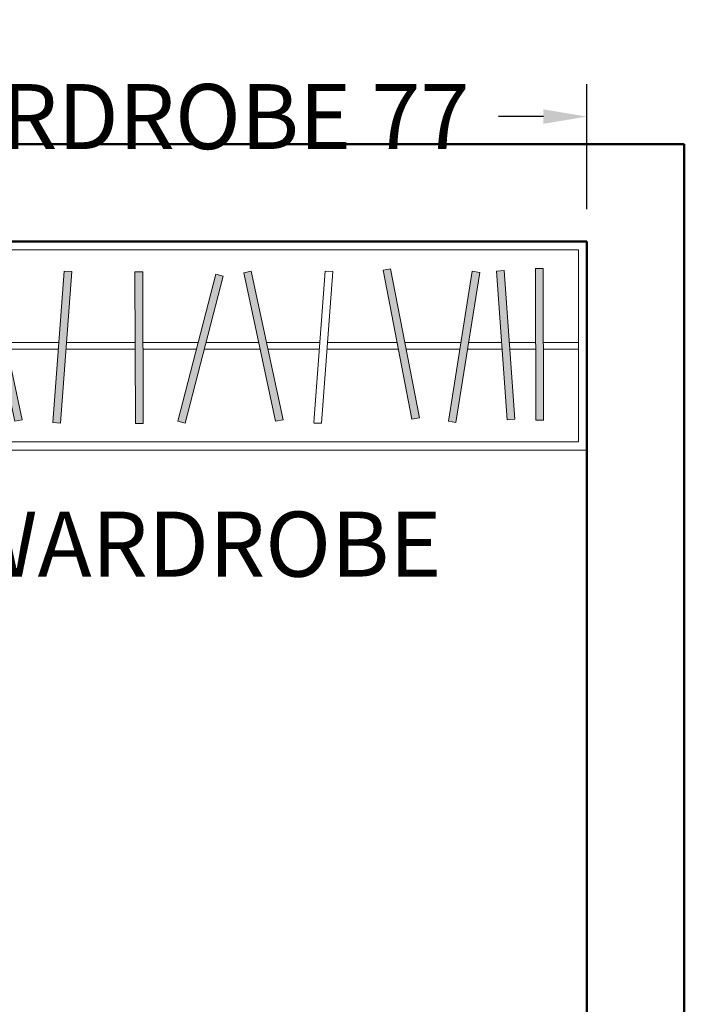
# Model space of a CAD drawing. Units: inches. Extents: x -466983 to 1020, y 324 to 318697.
# Tile 97 of 97: x 930 to 992, y 1006 to 1096. Entities that reach past the tile are written whole.
import ezdxf

# ---------------------------------------------------------------- set-up
doc = ezdxf.new("R2010")
doc.units = ezdxf.units.IN
doc.header["$MEASUREMENT"] = 0
for name, color, linetype, lineweight in [('A-ANNO-DIMS', 2, 'Continuous', 18), ('A-ANNO-TEXT', 7, 'Continuous', 18), ('A-FURN', 8, 'Continuous', 18), ('A-WALL', 7, 'Continuous', 50)]:
    doc.layers.add(name, color=color, linetype=linetype, lineweight=lineweight)
doc.styles.get("Standard").update_dxf_attribs({"font": 'arial.ttf'})
doc.dimstyles.get("Standard").update_dxf_attribs({"dimtxt": 6, "dimasz": 4, "dimexe": 3, "dimexo": 3, "dimgap": 0.09, "dimtad": 0, "dimtih": 1, "dimtoh": 1, "dimdec": 1, "dimzin": 0, "dimdsep": 46, "dimlunit": 3, "dimtxsty": 'Standard', "dimcen": 0.09, "dimadec": 0, "dimazin": 0, "dimtfac": 1, "dimtdec": 1, "dimtofl": 0, "dimtmove": 0, "dimatfit": 3, "dimfxl": 1, "dimtolj": 1, "dimtzin": 0, "dimarcsym": 0})

# ---------------------------------------------------------------- blocks, each defined once
blk = doc.blocks.new('Wardrobe 1.1')
h = blk.add_hatch(color=256)
h.dxf.hatch_style = 1
h.paths.add_polyline_path([(4623.63130591675, 1559.127828082639), (4605.452274823494, 1555.618178042687), (4674.43862754123, 1198.026895294012), (4692.617658634486, 1201.536545333964)])
h = blk.add_hatch(color=256)
h.dxf.hatch_style = 1
h.paths.add_polyline_path([(4989.37316691601, 1559.911022331437), (4970.858516418657, 1559.860704815934), (4971.798831744867, 1195.677017418713), (4990.313482242336, 1195.727334934216)])
h = blk.add_hatch(color=256)
h.dxf.hatch_style = 1
h.paths.add_polyline_path([(3151.282105115228, 1187.510288244974), (3169.796885531561, 1187.510288244974), (3168.856570205235, 1551.693975642194), (3150.341919707882, 1551.643658126692)])
h = blk.add_hatch(color=256)
h.dxf.hatch_style = 1
h.paths.add_polyline_path([(3361.868584936534, 1541.669378461711), (3343.939726713163, 1546.290077294676), (3253.002619132332, 1193.641406768397), (3270.931477355587, 1189.02070793549)])
h = blk.add_hatch(color=256)
h.dxf.hatch_style = 1
h.paths.add_polyline_path([(3403.891248248334, 1551.693975642194), (3385.376597750981, 1551.643658126692), (3386.316913077191, 1187.459970729471), (3404.831563574544, 1187.510288244974)])
h = blk.add_hatch(color=256)
h.dxf.hatch_style = 1
h.paths.add_polyline_path([(3596.9032629794, 1541.669378461711), (3578.974404756262, 1546.290077294676), (3488.037297175316, 1193.641406768397), (3505.966155398454, 1189.02070793549)])
h = blk.add_hatch(color=256)
h.dxf.hatch_style = 1
h.paths.add_polyline_path([(3664.213577620618, 1553.074679382599), (3646.111361609239, 1549.18821693327), (3722.509827192224, 1193.106882382172), (3740.612043203603, 1196.993344831501)])
h = blk.add_hatch(color=256)
h.dxf.hatch_style = 1
h.paths.add_polyline_path([(3813.833679657712, 1190.320201264565), (3832.296488257873, 1188.934736184298), (3859.597907476409, 1552.094859088468), (3841.135098876248, 1553.480324168735)])
h = blk.add_hatch(color=256)
h.dxf.hatch_style = 1
h.paths.add_polyline_path([(4029.392729275909, 1551.693975642194), (4010.878078778556, 1551.643658126692), (4011.818394104767, 1187.459970729471), (4030.333044602236, 1187.510288244974)])
h = blk.add_hatch(color=256)
h.dxf.hatch_style = 1
h.paths.add_polyline_path([(4222.404744007092, 1541.669378461711), (4204.475885783836, 1546.290077294676), (4113.538778203007, 1193.641406768397), (4131.467636426145, 1189.02070793549)])
h = blk.add_hatch(color=256)
h.dxf.hatch_style = 1
h.paths.add_polyline_path([(4348.011308219915, 1193.106882382172), (4366.113524231294, 1196.993344831501), (4289.715058648309, 1553.074679382599), (4271.612842636931, 1549.18821693327)])
h = blk.add_hatch(color=256)
h.dxf.hatch_style = 1
h.paths.add_polyline_path([(4837.600952654661, 1550.260731044678), (4819.316543353771, 1553.17194924514), (4762.004005428219, 1193.525017719703), (4780.288414729109, 1190.613799519242)])
h = blk.add_hatch(color=256)
h.dxf.hatch_style = 1
h.paths.add_polyline_path([(4895.873954488479, 1554.659198605851), (4877.410424046501, 1553.283386659738), (4902.671188982951, 1196.772307061869), (4921.13471942493, 1198.148119007923)])
at = {"ltscale": 5}
for p, q in [((3093.82979383441, 1124.111993690416), (3093.82979383441, 1624.111993690416)), ((3093.82979383441, 1624.111993690416), (5093.829793834409, 1624.111993690416)), ((5093.829793834409, 1624.111993690416), (5093.829793834409, 1124.111993690416)), ((5093.829793834409, 1124.111993690416), (3093.82979383441, 1124.111993690416))]:
    blk.add_line(p, q, dxfattribs=at)
for p, q in [((3113.82979383441, 1144.111993690416), (3113.82979383441, 1604.111993690416)), ((3113.82979383441, 1604.111993690416), (5073.829793834409, 1604.111993690416)), ((5073.829793834409, 1604.111993690416), (5073.829793834409, 1144.111993690416)), ((4623.63130591675, 1559.127828082639), (4605.452274823494, 1555.618178042687)), ((4692.617658634486, 1201.536545333964), (4623.63130591675, 1559.127828082639)), ((4989.37316691601, 1559.911022331437), (4970.858516418657, 1559.860704815934)), ((4970.858516418657, 1559.860704815934), (4971.798831744867, 1195.677017418713)), ((4990.313482242336, 1195.727334934216), (4989.37316691601, 1559.911022331437)), ((3168.856570205235, 1551.693975642194), (3150.341919707882, 1551.643658126692)), ((3150.341919707882, 1551.643658126692), (3151.282235034092, 1187.459970729471)), ((3169.796885531561, 1187.510288244974), (3168.856570205235, 1551.693975642194)), ((3343.939726713163, 1546.290077294676), (3253.002619132332, 1193.641406768397)), ((3270.931477355587, 1189.02070793549), (3361.868584936534, 1541.669378461711)), ((3361.868584936534, 1541.669378461711), (3343.939726713163, 1546.290077294676)), ((3403.891248248334, 1551.693975642194), (3385.376597750981, 1551.643658126692)), ((3385.376597750981, 1551.643658126692), (3386.316913077191, 1187.459970729471)), ((3404.831563574544, 1187.510288244974), (3403.891248248334, 1551.693975642194)), ((3578.974404756262, 1546.290077294676), (3488.037297175316, 1193.641406768397)), ((3505.966155398454, 1189.02070793549), (3596.9032629794, 1541.669378461711)), ((3596.9032629794, 1541.669378461711), (3578.974404756262, 1546.290077294676)), ((3664.213577620618, 1553.074679382599), (3646.111361609239, 1549.18821693327)), ((3646.111361609239, 1549.18821693327), (3722.509827192224, 1193.106882382172)), ((3740.612043203603, 1196.993344831501), (3664.213577620618, 1553.074679382599)), ((3841.135098876248, 1553.480324168735), (3813.833679657712, 1190.320201264565)), ((3832.296488257873, 1188.934736184298), (3859.597907476409, 1552.094859088468)), ((3859.597907476409, 1552.094859088468), (3841.135098876248, 1553.480324168735)), ((4029.392729275909, 1551.693975642194), (4010.878078778556, 1551.643658126692)), ((4010.878078778556, 1551.643658126692), (4011.818394104767, 1187.459970729471)), ((4030.333044602236, 1187.510288244974), (4029.392729275909, 1551.693975642194)), ((4204.475885783836, 1546.290077294676), (4113.538778203007, 1193.641406768397)), ((4131.467636426145, 1189.02070793549), (4222.404744007092, 1541.669378461711)), ((4222.404744007092, 1541.669378461711), (4204.475885783836, 1546.290077294676)), ((4289.715058648309, 1553.074679382599), (4271.612842636931, 1549.18821693327)), ((4271.612842636931, 1549.18821693327), (4348.011308219915, 1193.106882382172)), ((4366.113524231294, 1196.993344831501), (4289.715058648309, 1553.074679382599)), ((4605.452274823494, 1555.618178042687), (4674.43862754123, 1198.026895294012)), ((4819.316543353771, 1553.17194924514), (4762.004005428219, 1193.525017719703)), ((4780.288414729109, 1190.613799519242), (4837.600952654661, 1550.260731044678)), ((4837.600952654661, 1550.260731044678), (4819.316543353771, 1553.17194924514)), ((4895.873954488479, 1554.659198605851), (4877.410424046501, 1553.283386659738)), ((4877.410424046501, 1553.283386659738), (4902.671188982951, 1196.772307061869)), ((4921.13471942493, 1198.148119007923), (4895.873954488479, 1554.659198605851)), ((3150.779647227988, 1382.111993690416), (3113.82979383441, 1382.111993690416)), ((3301.603312885615, 1382.111993690416), (3169.294427644258, 1382.111993690416)), ((3301.603312885671, 1382.111993690416), (3169.294427644278, 1382.111993690416)), ((3385.814325271087, 1382.111993690416), (3320.723705409183, 1382.111993690416)), ((3536.63799092866, 1382.111993690416), (3404.329105687303, 1382.111993690416)), ((3536.637990928537, 1382.111993690416), (3404.329105687377, 1382.111993690416)), ((3681.958135513426, 1382.111993690416), (3555.75838345205, 1382.111993690416)), ((3681.958135513406, 1382.111993690416), (3555.758383452127, 1382.111993690416)), ((3828.252080240405, 1382.111993690416), (3700.894205307252, 1382.111993690416)), ((3828.252080240453, 1382.111993690416), (3700.894205307288, 1382.111993690416)), ((4011.315806298681, 1382.111993690416), (3846.819044447374, 1382.111993690416)), ((4162.139471956229, 1382.111993690416), (4029.830586714952, 1382.111993690416)), ((4307.459616541096, 1382.111993690416), (4181.259864479818, 1382.111993690416)), ((4453.753561268143, 1382.111993690416), (4326.395686334979, 1382.111993690416)), ((4638.925011464094, 1382.111993690416), (4472.320525475011, 1382.111993690416)), ((4792.056807955193, 1382.111993690416), (4657.781122696752, 1382.111993690416)), ((4889.538855865531, 1382.111993690416), (4810.805142536459, 1382.111993690416)), ((4971.317460196375, 1382.111993690416), (4908.099870128257, 1382.111993690416)), ((5073.829793834409, 1382.111993690416), (4989.832240612645, 1382.111993690416)), ((3150.820958922443, 1366.111993690417), (3113.82979383441, 1366.111993690416)), ((3297.477411264826, 1366.111993690417), (3169.335739338719, 1366.111993690417)), ((3297.477411264836, 1366.111993690416), (3169.33573933882, 1366.111993690416)), ((3385.855636965543, 1366.111993690416), (3316.597803788389, 1366.111993690416)), ((3532.512089307866, 1366.111993690416), (3404.370417381759, 1366.111993690416)), ((3532.512089307935, 1366.111993690416), (3404.370417381687, 1366.111993690416)), ((3685.390990119154, 1366.111993690416), (3551.632481831255, 1366.111993690417)), ((3685.390990119244, 1366.111993690416), (3551.632481831408, 1366.111993690416)), ((3827.049242483872, 1366.111993690416), (3704.32705991298, 1366.111993690416)), ((3827.049242483967, 1366.111993690416), (3704.327059913011, 1366.111993690416)), ((4011.357117993108, 1366.111993690416), (3845.61620669084, 1366.111993690416)), ((4158.013570335509, 1366.111993690416), (4029.871898409377, 1366.111993690416)), ((4310.892471146819, 1366.111993690416), (4177.133962858983, 1366.111993690416)), ((4452.550723511541, 1366.111993690416), (4329.828540940702, 1366.111993690416)), ((4642.011724414702, 1366.111993690416), (4471.117687718526, 1366.111993690416)), ((4789.507083415918, 1366.111993690416), (4660.867835647359, 1366.111993690416)), ((4890.672543602346, 1366.111993690416), (4808.255417997067, 1366.111993690416)), ((4971.3587718908, 1366.111993690416), (4909.233557865072, 1366.111993690416)), ((5073.829793834409, 1366.111993690416), (4989.873552307186, 1366.111993690416)), ((3169.796885531561, 1187.510288244974), (3151.282105115229, 1187.510288244974)), ((3253.002619132332, 1193.641406768397), (3270.931477355587, 1189.02070793549)), ((3404.831563574544, 1187.510288244974), (3386.316913077191, 1187.459970729471)), ((3488.037297175316, 1193.641406768397), (3505.966155398454, 1189.02070793549)), ((3722.509827192224, 1193.106882382172), (3740.612043203603, 1196.993344831501)), ((3832.296488257873, 1188.934736184298), (3813.833679657712, 1190.320201264565)), ((4030.333044602236, 1187.510288244974), (4011.818394104767, 1187.459970729471)), ((4113.538778203007, 1193.641406768397), (4131.467636426145, 1189.02070793549)), ((4348.011308219915, 1193.106882382172), (4366.113524231294, 1196.993344831501)), ((4674.43862754123, 1198.026895294012), (4692.617658634486, 1201.536545333964)), ((4762.004005428219, 1193.525017719703), (4780.288414729109, 1190.613799519242)), ((4902.671188982951, 1196.772307061869), (4921.13471942493, 1198.148119007923)), ((4971.798831744867, 1195.677017418713), (4990.313482242336, 1195.727334934216)), ((5073.829793834409, 1144.111993690416), (3113.82979383441, 1144.111993690416))]:
    blk.add_line(p, q)
blk.add_lwpolyline([(4439.335160685403, 1190.320201264565), (4466.63657990394, 1553.480324168735), (4485.0993885041, 1552.094859088468), (4457.797969285564, 1188.934736184298), (4439.231005078596, 1188.934736184298)])
blk = doc.blocks.new('*D85')
at = {"layer": 'A-ANNO-DIMS', "color": 0, "lineweight": -2, "transparency": 16777216}
for p, q in [((905.8056775209042, 1078.937732818421), (905.8056775209042, 1090.487732818421)), ((982.805677520904, 1078.937732818421), (982.805677520904, 1090.487732818421)), ((909.805677520904, 1087.487732818421), (913.9496475072615, 1087.487732818421)), ((978.805677520904, 1087.487732818421), (974.6617075345467, 1087.487732818421))]:
    blk.add_line(p, q, dxfattribs=at)
at = {"layer": 'A-ANNO-DIMS', "color": 0, "transparency": 16777216}
for points in [[(909.805677520904, 1088.154399485087), (909.805677520904, 1086.821066151754), (905.8056775209042, 1087.487732818421)], [(978.805677520904, 1088.154399485087), (978.805677520904, 1086.821066151754), (982.805677520904, 1087.487732818421)]]:
    blk.add_solid(points, dxfattribs=at)
at = {"layer": 'Defpoints', "color": 0, "transparency": 16777216}
for p in [(982.805677520904, 1087.487732818421), (905.8056775209042, 1075.937732818421), (982.805677520904, 1075.937732818421)]:
    blk.add_point(p, dxfattribs=at)
at = {"layer": 'A-ANNO-DIMS', "color": 0, "transparency": 16777216, "insert": (944.305677520904, 1087.487732818421), "char_height": 6, "attachment_point": 5}
blk.add_mtext('\\A1;WARDROBE 77', dxfattribs=at)
blk = doc.blocks.new('*D88')
at = {"layer": 'A-ANNO-DIMS', "color": 0, "lineweight": -2, "transparency": 16777216}
for p, q in [((949.3303071758708, 990.0607643795369), (949.3303071758708, 1003.232436010027)), ((982.3282315749892, 990.0607643795369), (982.3282315749892, 1003.232436010027)), ((945.3303071758706, 1000.232436010027), (941.3303071758708, 1000.232436010027)), ((986.3282315749891, 1000.232436010027), (990.3282315749892, 1000.232436010027))]:
    blk.add_line(p, q, dxfattribs=at)
at = {"layer": 'A-ANNO-DIMS', "color": 0, "transparency": 16777216}
for points in [[(945.3303071758706, 1000.899102676694), (945.3303071758706, 999.5657693433604), (949.3303071758708, 1000.232436010027)], [(986.3282315749891, 1000.899102676694), (986.3282315749891, 999.5657693433604), (982.3282315749892, 1000.232436010027)]]:
    blk.add_solid(points, dxfattribs=at)
at = {"layer": 'Defpoints', "color": 0, "transparency": 16777216}
for p in [(949.3303071758708, 1000.232436010027), (949.3303071758708, 987.060764379537), (982.3282315749892, 987.060764379537)]:
    blk.add_point(p, dxfattribs=at)
at = {"layer": 'A-ANNO-DIMS', "color": 0, "transparency": 16777216, "insert": (965.8292693754299, 1000.232436010027), "char_height": 6, "attachment_point": 5}
blk.add_mtext('\\A1;33 TYP.', dxfattribs=at)

msp = doc.modelspace()

# ---------------------------------------------------------------- linework, layer by layer
at = {"layer": 'A-WALL'}
for p, q in [((391.8056775209043, 1084.937732818421), (991.8056775209043, 1084.937732818421)), ((991.8056775209043, 1084.937732818421), (991.8056775209043, 364.9377328184219)), ((813.8056775209042, 1075.937732818422), (982.805677520904, 1075.937732818422)), ((982.805677520904, 1075.937732818422), (982.805677520904, 828.9377328184212))]:
    msp.add_line(p, q, dxfattribs=at)

# ---------------------------------------------------------------- block references
at = {"layer": 'A-FURN', "xscale": 0.0385, "yscale": 0.0385, "zscale": 0.0385}
msp.add_blockref('Wardrobe 1.1', (786.6932304582793, 1013.40942106134), dxfattribs=at)

# ---------------------------------------------------------------- texts
at = {"layer": 'A-ANNO-TEXT', "insert": (832.3947444543959, 1051.000964560194), "char_height": 6, "attachment_point": 1}
msp.add_mtext_dynamic_manual_height_columns('\\pxqc;WARDROBE', width=229.5582916082931, gutter_width=1, heights=[0], dxfattribs=at)

# ---------------------------------------------------------------- dimensions: what is measured, and where the dimension line sits
at = {"layer": 'A-ANNO-DIMS'}
dim = msp.add_linear_dim(base=(982.805677520904, 1087.487732818421), p1=(905.8056775209042, 1075.937732818421), p2=(982.805677520904, 1075.937732818421), text='WARDROBE <>', dimstyle='Standard', override={"dimdec": 0, "dimlfac": 1, "dimrnd": 0, "dimzin": 0, "dimdsep": 46, "dimlunit": 2}, dxfattribs=at)
dim.commit()
dim.dimension.update_dxf_attribs({"geometry": '*D85', "text_midpoint": (944.305677520904, 1087.487732818421)})
dim = msp.add_linear_dim(base=(949.3303071758708, 1000.232436010027), p1=(982.3282315749892, 987.060764379537), p2=(949.3303071758708, 987.060764379537), angle=180, text='<> TYP.', dimstyle='Standard', override={"dimdec": 0, "dimlfac": 1, "dimrnd": 0, "dimzin": 0, "dimdsep": 46, "dimlunit": 2}, dxfattribs=at)
dim.commit()
dim.dimension.update_dxf_attribs({"geometry": '*D88', "text_midpoint": (965.8292693754299, 1000.232436010027)})

doc.saveas('drawing.dxf')
